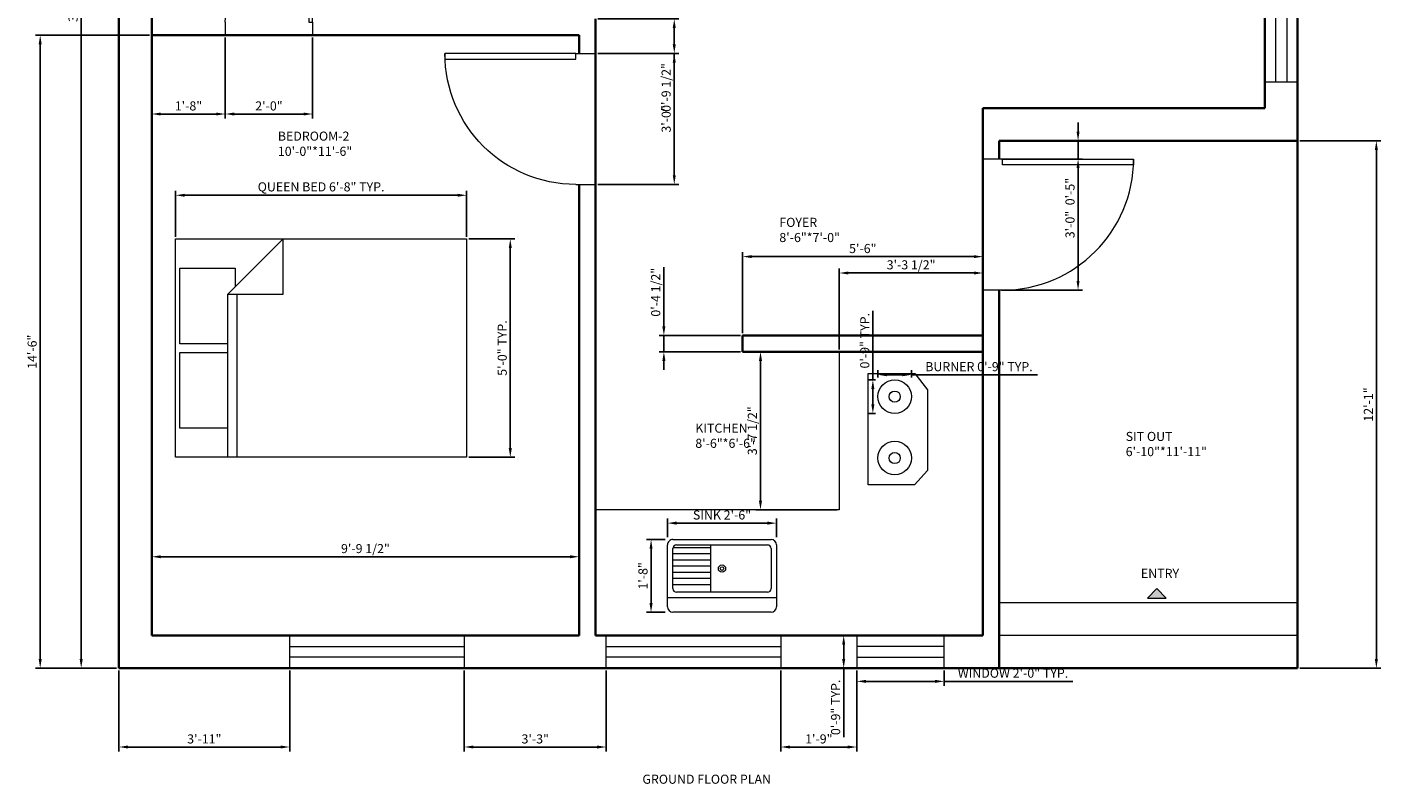
# Model space of a CAD drawing. Units: inches. Extents: x 2721 to 3093, y 1944 to 2371.
# Tile 1 of 2: x 2721 to 3093, y 1944 to 2152. Entities that reach past the tile are written whole.
import ezdxf

# ---------------------------------------------------------------- set-up
doc = ezdxf.new("R2010")
doc.units = ezdxf.units.IN
for name, color, linetype, lineweight in [('A-ANNO-DIMS', 2, 'Continuous', 18), ('A-ANNO-SYMB', 7, 'Continuous', 13), ('A-ANNO-SYMB-PATT', 7, 'Continuous', 13), ('A-ANNO-TEXT', 7, 'Continuous', 18), ('A-AREA-IDEN', 7, 'Continuous', 18), ('A-DOOR', 3, 'Continuous', 18), ('A-EQPM', 8, 'Continuous', 18), ('A-FLOR-CASE', 8, 'Continuous', 20), ('A-FLOR-FIXT', 8, 'Continuous', 18), ('A-FLOR-FIXT-PATT', 8, 'Continuous', 13), ('A-FLOR-STRS', 7, 'Continuous', 20), ('A-FURN', 9, 'Continuous', 18), ('A-GLAZ', 4, 'Continuous', 18), ('A-WALL', 7, 'Continuous', 35)]:
    doc.layers.add(name, color=color, linetype=linetype, lineweight=lineweight)
doc.styles.get("Standard").update_dxf_attribs({"font": 'arial.ttf'})
doc.dimstyles.new('ISO-25', dxfattribs={"dimtxt": 2.5, "dimasz": 2.5, "dimexe": 1.25, "dimexo": 0.625, "dimtad": 1, "dimdec": 1, "dimlunit": 3, "dimtxsty": 'Standard', "dimcen": 2.5, "dimadec": 0, "dimazin": 0, "dimtfac": 1, "dimtdec": 1, "dimtmove": 0, "dimatfit": 3, "dimfxl": 1, "dimarcsym": 0})

# ---------------------------------------------------------------- blocks, each defined once
blk = doc.blocks.new('*U2')
for p, q in [((0, 0), (0, -6)), ((40, 0), (40, -6))]:
    blk.add_line(p, q)
blk.add_lwpolyline([(0, 0), (0, 40), (1.75, 40), (1.75, 0)], close=True)
blk.add_arc((0, 0), 40, 0, 90)
blk = doc.blocks.new('Bed - Queen')
for p, q in [((0, -80.00003), (0, 0)), ((0, 0), (59.99999, 0)), ((59.99999, 0), (59.99999, -80.00003)), ((7.99999, -1.2), (28.79998, -1.2)), ((7.99999, -14.4), (7.99999, -1.2)), ((28.79998, -1.2), (28.79998, -14.4)), ((31.19999, -1.2), (51.99999, -1.2)), ((31.19999, -14.4), (31.19999, -1.2)), ((51.99999, -1.2), (51.99999, -16.4)), ((0, -14.4), (44.8, -14.4)), ((59.99999, -29.6), (44.8, -14.4)), ((44.8, -14.4), (44.8, -29.6)), ((44.8, -16.8), (0, -16.8)), ((51.99999, -16.4), (46.79936, -16.4)), ((44.8, -29.6), (59.99999, -29.6)), ((59.99999, -80.00003), (0, -80.00003))]:
    blk.add_line(p, q)
blk = doc.blocks.new('Sink-single - 30 in top')
blk.add_line((-15, -3.999996), (15, -3.999996))
for points in [[(-13.5, 0), (13.5, 0)], [(-15, -18.499996), (-15, -1.5)], [(15, -1.5), (15, -18.499996)], [(-13.5, -17.499996), (-13.5, -6.499996)], [(-12.5, -5.499996), (12.5, -5.499996)], [(13.5, -6.499996), (13.5, -17.499996)], [(12.5, -18.499996), (-12.5, -18.499996)], [(13.5, -19.999996), (-13.5, -19.999996)]]:
    blk.add_lwpolyline(points)
for radius in [1, 0.5]:
    blk.add_circle((0, -11.999996), radius)
for centre, radius, start, end in [((-13.5, -1.5), 1.5, 90, 180), ((13.5, -1.5), 1.5, 0, 90), ((-12.5, -6.499996), 1, 90, 180), ((12.5, -6.499996), 1, 0, 90), ((-13.5, -18.499996), 1.5, 180, 270), ((-12.5, -17.499996), 1, 180, 270), ((12.5, -17.499996), 1, 270, 0), ((13.5, -18.499996), 1.5, 270, 0)]:
    blk.add_arc(centre, radius, start, end)
blk = doc.blocks.new('*D7')
at = {"layer": 'A-ANNO-DIMS', "color": 0, "lineweight": -2, "transparency": 16777216}
for p, q in [((2745.17, 2336.18), (2734.17, 2336.18)), ((2735.42, 2333.68), (2735.42, 1978.68)), ((2745.17, 1976.18), (2734.17, 1976.18))]:
    blk.add_line(p, q, dxfattribs=at)
at = {"layer": 'A-ANNO-DIMS', "color": 0, "transparency": 16777216}
for points in [[(2735, 2333.68), (2735.84, 2333.68), (2735.42, 2336.18)], [(2735, 1978.68), (2735.84, 1978.68), (2735.42, 1976.18)]]:
    blk.add_solid(points, dxfattribs=at)
at = {"layer": 'Defpoints', "color": 0, "transparency": 16777216}
for p in [(2745.8, 2336.18), (2735.42, 1976.18), (2745.8, 1976.18)]:
    blk.add_point(p, dxfattribs=at)
at = {"layer": 'A-ANNO-DIMS', "color": 0, "transparency": 16777216, "insert": (2733.52, 2156.18), "char_height": 2.5, "attachment_point": 5, "rotation": 90}
blk.add_mtext("30'", dxfattribs=at)
blk = doc.blocks.new('WIN-48IN')
for p, q in [((0, 9), (48, 9)), ((0, 0), (0, 9)), ((48, 9), (48, 0)), ((0, 6), (48, 6)), ((48, 3), (0, 3)), ((48, 0), (0, 0))]:
    blk.add_line(p, q)
blk = doc.blocks.new('WIN-24IN')
for p, q in [((9, 24), (0, 24)), ((0, 24), (0, 0)), ((3, 24), (3, 0)), ((6, 0), (6, 24)), ((9, 0), (9, 24)), ((0, 0), (9, 0))]:
    blk.add_line(p, q)
blk = doc.blocks.new('COOKTOP-BURNER')
for radius in [4.62, 1.54]:
    blk.add_circle((4.62, 4.62), radius)
blk = doc.blocks.new('*D13')
at = {"layer": 'A-ANNO-DIMS', "color": 0, "lineweight": -2, "transparency": 16777216}
for p, q in [((2948.62, 1975.55), (2948.62, 1971.33)), ((2951.12, 1972.58), (2970.12, 1972.58)), ((2972.62, 1975.55), (2972.62, 1971.33)), ((2972.62, 1972.58), (3008, 1972.58))]:
    blk.add_line(p, q, dxfattribs=at)
at = {"layer": 'A-ANNO-DIMS', "color": 0, "transparency": 16777216}
for points in [[(2951.12, 1972.99), (2951.12, 1972.16), (2948.62, 1972.58)], [(2970.12, 1972.99), (2970.12, 1972.16), (2972.62, 1972.58)]]:
    blk.add_solid(points, dxfattribs=at)
at = {"layer": 'Defpoints', "color": 0, "transparency": 16777216}
for p in [(2948.62, 1976.18), (2972.62, 1976.18), (2972.62, 1972.58)]:
    blk.add_point(p, dxfattribs=at)
at = {"layer": 'A-ANNO-DIMS', "color": 0, "transparency": 16777216, "insert": (2991.56, 1974.5), "char_height": 2.5, "attachment_point": 5}
blk.add_mtext('WINDOW 2\'-0" TYP.', dxfattribs=at)
blk = doc.blocks.new('*D14')
at = {"layer": 'A-ANNO-DIMS', "color": 0, "lineweight": -2, "transparency": 16777216}
for p, q in [((2947.99, 1985.18), (2943.77, 1985.18)), ((2945.02, 1982.68), (2945.02, 1978.68)), ((2947.99, 1976.18), (2943.77, 1976.18)), ((2945.02, 1976.18), (2945.02, 1957.19))]:
    blk.add_line(p, q, dxfattribs=at)
at = {"layer": 'A-ANNO-DIMS', "color": 0, "transparency": 16777216}
for points in [[(2944.6, 1982.68), (2945.43, 1982.68), (2945.02, 1985.18)], [(2944.6, 1978.68), (2945.43, 1978.68), (2945.02, 1976.18)]]:
    blk.add_solid(points, dxfattribs=at)
at = {"layer": 'Defpoints', "color": 0, "transparency": 16777216}
for p in [(2948.62, 1985.18), (2945.02, 1976.18), (2948.62, 1976.18)]:
    blk.add_point(p, dxfattribs=at)
at = {"layer": 'A-ANNO-DIMS', "color": 0, "transparency": 16777216, "insert": (2943.12, 1965.43), "char_height": 2.5, "attachment_point": 5, "rotation": 90}
blk.add_mtext('0\'-9" TYP.', dxfattribs=at)
blk = doc.blocks.new('*D15')
at = {"layer": 'A-ANNO-DIMS', "color": 0, "lineweight": -2, "transparency": 16777216}
for p, q in [((2761.37, 2094.81), (2761.37, 2107.44)), ((2841.37, 2094.81), (2841.37, 2107.44)), ((2838.87, 2106.19), (2763.87, 2106.19))]:
    blk.add_line(p, q, dxfattribs=at)
at = {"layer": 'A-ANNO-DIMS', "color": 0, "transparency": 16777216}
for points in [[(2763.87, 2106.61), (2763.87, 2105.77), (2761.37, 2106.19)], [(2838.87, 2106.61), (2838.87, 2105.77), (2841.37, 2106.19)]]:
    blk.add_solid(points, dxfattribs=at)
at = {"layer": 'Defpoints', "color": 0, "transparency": 16777216}
for p in [(2761.37, 2106.19), (2761.37, 2094.19), (2841.37, 2094.19)]:
    blk.add_point(p, dxfattribs=at)
at = {"layer": 'A-ANNO-DIMS', "color": 0, "transparency": 16777216, "insert": (2801.37, 2108.18), "char_height": 2.5, "attachment_point": 5}
blk.add_mtext('QUEEN BED 6\'-8" TYP.', dxfattribs=at)
blk = doc.blocks.new('*D16')
at = {"layer": 'A-ANNO-DIMS', "color": 0, "lineweight": -2, "transparency": 16777216}
for p, q in [((2842, 2094.19), (2854.62, 2094.19)), ((2853.37, 2036.69), (2853.37, 2091.69)), ((2842, 2034.19), (2854.62, 2034.19))]:
    blk.add_line(p, q, dxfattribs=at)
at = {"layer": 'A-ANNO-DIMS', "color": 0, "transparency": 16777216}
for points in [[(2852.95, 2091.69), (2853.79, 2091.69), (2853.37, 2094.19)], [(2852.95, 2036.69), (2853.79, 2036.69), (2853.37, 2034.19)]]:
    blk.add_solid(points, dxfattribs=at)
at = {"layer": 'Defpoints', "color": 0, "transparency": 16777216}
for p in [(2841.37, 2094.19), (2853.37, 2094.19), (2841.37, 2034.19)]:
    blk.add_point(p, dxfattribs=at)
at = {"layer": 'A-ANNO-DIMS', "color": 0, "transparency": 16777216, "insert": (2851.47, 2064.19), "char_height": 2.5, "attachment_point": 5, "rotation": 90}
blk.add_mtext('5\'-0" TYP.', dxfattribs=at)
blk = doc.blocks.new('*D19')
at = {"layer": 'A-ANNO-DIMS', "color": 0, "lineweight": -2, "transparency": 16777216}
for p, q in [((2954.43, 2056.09), (2954.43, 2058.1)), ((2963.66, 2056.09), (2963.66, 2058.1)), ((2956.93, 2056.85), (2961.16, 2056.85)), ((2963.66, 2056.85), (2998.26, 2056.85))]:
    blk.add_line(p, q, dxfattribs=at)
at = {"layer": 'A-ANNO-DIMS', "color": 0, "transparency": 16777216}
for points in [[(2956.93, 2057.27), (2956.93, 2056.44), (2954.43, 2056.85)], [(2961.16, 2057.27), (2961.16, 2056.44), (2963.66, 2056.85)]]:
    blk.add_solid(points, dxfattribs=at)
at = {"layer": 'Defpoints', "color": 0, "transparency": 16777216}
for p in [(2954.43, 2055.47), (2963.66, 2056.85), (2963.66, 2055.47)]:
    blk.add_point(p, dxfattribs=at)
at = {"layer": 'A-ANNO-DIMS', "color": 0, "transparency": 16777216, "insert": (2982.21, 2058.76), "char_height": 2.5, "attachment_point": 5}
blk.add_mtext('BURNER 0\'-9" TYP.', dxfattribs=at)
blk = doc.blocks.new('*D20')
at = {"layer": 'A-ANNO-DIMS', "color": 0, "lineweight": -2, "transparency": 16777216}
for p, q in [((2953.04, 2055.47), (2953.04, 2074.46)), ((2953.8, 2055.47), (2951.79, 2055.47)), ((2953.04, 2048.73), (2953.04, 2052.97)), ((2953.8, 2046.23), (2951.79, 2046.23))]:
    blk.add_line(p, q, dxfattribs=at)
at = {"layer": 'A-ANNO-DIMS', "color": 0, "transparency": 16777216}
for points in [[(2952.62, 2052.97), (2953.46, 2052.97), (2953.04, 2055.47)], [(2952.62, 2048.73), (2953.46, 2048.73), (2953.04, 2046.23)]]:
    blk.add_solid(points, dxfattribs=at)
at = {"layer": 'Defpoints', "color": 0, "transparency": 16777216}
for p in [(2953.04, 2055.47), (2954.43, 2055.47), (2954.43, 2046.23)]:
    blk.add_point(p, dxfattribs=at)
at = {"layer": 'A-ANNO-DIMS', "color": 0, "transparency": 16777216, "insert": (2951.14, 2066.21), "char_height": 2.5, "attachment_point": 5, "rotation": 90}
blk.add_mtext('0\'-9" TYP.', dxfattribs=at)
blk = doc.blocks.new('*D21')
at = {"layer": 'A-ANNO-DIMS', "color": 0, "lineweight": -2, "transparency": 16777216}
for p, q in [((2896.57, 2012.2), (2896.57, 2017.32)), ((2926.57, 2012.2), (2926.57, 2017.32)), ((2924.07, 2016.07), (2899.07, 2016.07))]:
    blk.add_line(p, q, dxfattribs=at)
at = {"layer": 'A-ANNO-DIMS', "color": 0, "transparency": 16777216}
for points in [[(2899.07, 2016.49), (2899.07, 2015.65), (2896.57, 2016.07)], [(2924.07, 2016.49), (2924.07, 2015.65), (2926.57, 2016.07)]]:
    blk.add_solid(points, dxfattribs=at)
at = {"layer": 'Defpoints', "color": 0, "transparency": 16777216}
for p in [(2896.57, 2016.07), (2896.57, 2011.57), (2926.57, 2011.57)]:
    blk.add_point(p, dxfattribs=at)
at = {"layer": 'A-ANNO-DIMS', "color": 0, "transparency": 16777216, "insert": (2911.57, 2017.99), "char_height": 2.5, "attachment_point": 5}
blk.add_mtext('SINK 2\'-6"', dxfattribs=at)
blk = doc.blocks.new('*D22')
at = {"layer": 'A-ANNO-DIMS', "color": 0, "lineweight": -2, "transparency": 16777216}
for p, q in [((2895.94, 2011.57), (2890.82, 2011.57)), ((2892.07, 2009.07), (2892.07, 1994.07)), ((2895.94, 1991.57), (2890.82, 1991.57))]:
    blk.add_line(p, q, dxfattribs=at)
at = {"layer": 'A-ANNO-DIMS', "color": 0, "transparency": 16777216}
for points in [[(2891.65, 2009.07), (2892.48, 2009.07), (2892.07, 2011.57)], [(2891.65, 1994.07), (2892.48, 1994.07), (2892.07, 1991.57)]]:
    blk.add_solid(points, dxfattribs=at)
at = {"layer": 'Defpoints', "color": 0, "transparency": 16777216}
for p in [(2896.57, 2011.57), (2892.07, 1991.57), (2896.57, 1991.57)]:
    blk.add_point(p, dxfattribs=at)
at = {"layer": 'A-ANNO-DIMS', "color": 0, "transparency": 16777216, "insert": (2890.17, 2001.57), "char_height": 2.5, "attachment_point": 5, "rotation": 90}
blk.add_mtext('1\'-8"', dxfattribs=at)
blk = doc.blocks.new('*D25')
at = {"layer": 'A-ANNO-DIMS', "color": 0, "lineweight": -2, "transparency": 16777216}
for p, q in [((2745.8, 1975.55), (2745.8, 1953.28)), ((2792.73, 1975.55), (2792.73, 1953.28)), ((2790.23, 1954.53), (2748.3, 1954.53))]:
    blk.add_line(p, q, dxfattribs=at)
at = {"layer": 'A-ANNO-DIMS', "color": 0, "transparency": 16777216}
for points in [[(2748.3, 1954.94), (2748.3, 1954.11), (2745.8, 1954.53)], [(2790.23, 1954.94), (2790.23, 1954.11), (2792.73, 1954.53)]]:
    blk.add_solid(points, dxfattribs=at)
at = {"layer": 'Defpoints', "color": 0, "transparency": 16777216}
for p in [(2745.8, 1976.18), (2792.73, 1976.18), (2745.8, 1954.53)]:
    blk.add_point(p, dxfattribs=at)
at = {"layer": 'A-ANNO-DIMS', "color": 0, "transparency": 16777216, "insert": (2769.26, 1956.43), "char_height": 2.5, "attachment_point": 5}
blk.add_mtext('3\'-11"', dxfattribs=at)
blk = doc.blocks.new('*D26')
at = {"layer": 'A-ANNO-DIMS', "color": 0, "lineweight": -2, "transparency": 16777216}
for p, q in [((2840.73, 1975.55), (2840.73, 1953.28)), ((2879.73, 1975.55), (2879.73, 1953.28)), ((2877.23, 1954.53), (2843.23, 1954.53))]:
    blk.add_line(p, q, dxfattribs=at)
at = {"layer": 'A-ANNO-DIMS', "color": 0, "transparency": 16777216}
for points in [[(2843.23, 1954.94), (2843.23, 1954.11), (2840.73, 1954.53)], [(2877.23, 1954.94), (2877.23, 1954.11), (2879.73, 1954.53)]]:
    blk.add_solid(points, dxfattribs=at)
at = {"layer": 'Defpoints', "color": 0, "transparency": 16777216}
for p in [(2840.73, 1976.18), (2879.73, 1976.18), (2840.73, 1954.53)]:
    blk.add_point(p, dxfattribs=at)
at = {"layer": 'A-ANNO-DIMS', "color": 0, "transparency": 16777216, "insert": (2860.23, 1956.43), "char_height": 2.5, "attachment_point": 5}
blk.add_mtext('3\'-3"', dxfattribs=at)
blk = doc.blocks.new('*D27')
at = {"layer": 'A-ANNO-DIMS', "color": 0, "lineweight": -2, "transparency": 16777216}
for p, q in [((2927.73, 1975.55), (2927.73, 1953.28)), ((2948.62, 1975.55), (2948.62, 1953.28)), ((2946.12, 1954.53), (2930.23, 1954.53))]:
    blk.add_line(p, q, dxfattribs=at)
at = {"layer": 'A-ANNO-DIMS', "color": 0, "transparency": 16777216}
for points in [[(2930.23, 1954.94), (2930.23, 1954.11), (2927.73, 1954.53)], [(2946.12, 1954.94), (2946.12, 1954.11), (2948.62, 1954.53)]]:
    blk.add_solid(points, dxfattribs=at)
at = {"layer": 'Defpoints', "color": 0, "transparency": 16777216}
for p in [(2927.73, 1976.18), (2948.62, 1976.18), (2927.73, 1954.53)]:
    blk.add_point(p, dxfattribs=at)
at = {"layer": 'A-ANNO-DIMS', "color": 0, "transparency": 16777216, "insert": (2938.18, 1956.43), "char_height": 2.5, "attachment_point": 5}
blk.add_mtext('1\'-9"', dxfattribs=at)
blk = doc.blocks.new('*D32')
at = {"layer": 'A-ANNO-DIMS', "color": 0, "lineweight": -2, "transparency": 16777216}
for p, q in [((2988.42, 2116.15), (3010.7, 2116.15)), ((3009.45, 2113.65), (3009.45, 2082.65)), ((2988.42, 2080.15), (3010.7, 2080.15))]:
    blk.add_line(p, q, dxfattribs=at)
at = {"layer": 'A-ANNO-DIMS', "color": 0, "transparency": 16777216}
for points in [[(3009.03, 2113.65), (3009.86, 2113.65), (3009.45, 2116.15)], [(3009.03, 2082.65), (3009.86, 2082.65), (3009.45, 2080.15)]]:
    blk.add_solid(points, dxfattribs=at)
at = {"layer": 'Defpoints', "color": 0, "transparency": 16777216}
for p in [(2987.8, 2116.15), (2987.8, 2080.15), (3009.45, 2080.15)]:
    blk.add_point(p, dxfattribs=at)
at = {"layer": 'A-ANNO-DIMS', "color": 0, "transparency": 16777216, "insert": (3007.55, 2098.15), "char_height": 2.5, "attachment_point": 5, "rotation": 90}
blk.add_mtext('3\'-0"', dxfattribs=at)
blk = doc.blocks.new('*D33')
at = {"layer": 'A-ANNO-DIMS', "color": 0, "lineweight": -2, "transparency": 16777216}
for p, q in [((2775.03, 2149.55), (2775.03, 2127.28)), ((2799.03, 2149.55), (2799.03, 2127.28)), ((2796.53, 2128.53), (2777.53, 2128.53))]:
    blk.add_line(p, q, dxfattribs=at)
at = {"layer": 'A-ANNO-DIMS', "color": 0, "transparency": 16777216}
for points in [[(2777.53, 2128.94), (2777.53, 2128.11), (2775.03, 2128.53)], [(2796.53, 2128.94), (2796.53, 2128.11), (2799.03, 2128.53)]]:
    blk.add_solid(points, dxfattribs=at)
at = {"layer": 'Defpoints', "color": 0, "transparency": 16777216}
for p in [(2775.03, 2150.18), (2799.03, 2150.18), (2775.03, 2128.53)]:
    blk.add_point(p, dxfattribs=at)
at = {"layer": 'A-ANNO-DIMS', "color": 0, "transparency": 16777216, "insert": (2787.03, 2130.43), "char_height": 2.5, "attachment_point": 5}
blk.add_mtext('2\'-0"', dxfattribs=at)
blk = doc.blocks.new('*D37')
at = {"layer": 'A-ANNO-DIMS', "color": 0, "lineweight": -2, "transparency": 16777216}
for p, q in [((2877.42, 2145.18), (2899.7, 2145.18)), ((2898.45, 2142.68), (2898.45, 2111.68)), ((2877.42, 2109.18), (2899.7, 2109.18))]:
    blk.add_line(p, q, dxfattribs=at)
at = {"layer": 'A-ANNO-DIMS', "color": 0, "transparency": 16777216}
for points in [[(2898.03, 2142.68), (2898.86, 2142.68), (2898.45, 2145.18)], [(2898.03, 2111.68), (2898.86, 2111.68), (2898.45, 2109.18)]]:
    blk.add_solid(points, dxfattribs=at)
at = {"layer": 'Defpoints', "color": 0, "transparency": 16777216}
for p in [(2876.8, 2145.18), (2876.8, 2109.18), (2898.45, 2109.18)]:
    blk.add_point(p, dxfattribs=at)
at = {"layer": 'A-ANNO-DIMS', "color": 0, "transparency": 16777216, "insert": (2896.55, 2127.18), "char_height": 2.5, "attachment_point": 5, "rotation": 90}
blk.add_mtext('3\'-0"', dxfattribs=at)
blk = doc.blocks.new('*D38')
at = {"layer": 'A-ANNO-DIMS', "color": 0, "lineweight": -2, "transparency": 16777216}
for p, q in [((3070.42, 2121.18), (3092.7, 2121.18)), ((3091.45, 2118.68), (3091.45, 1978.68)), ((3070.42, 1976.18), (3092.7, 1976.18))]:
    blk.add_line(p, q, dxfattribs=at)
at = {"layer": 'A-ANNO-DIMS', "color": 0, "transparency": 16777216}
for points in [[(3091.03, 2118.68), (3091.86, 2118.68), (3091.45, 2121.18)], [(3091.03, 1978.68), (3091.86, 1978.68), (3091.45, 1976.18)]]:
    blk.add_solid(points, dxfattribs=at)
at = {"layer": 'Defpoints', "color": 0, "transparency": 16777216}
for p in [(3069.8, 2121.18), (3069.8, 1976.18), (3091.45, 1976.18)]:
    blk.add_point(p, dxfattribs=at)
at = {"layer": 'A-ANNO-DIMS', "color": 0, "transparency": 16777216, "insert": (3089.57, 2048.68), "char_height": 2.5, "attachment_point": 5, "rotation": 90}
blk.add_mtext('12\'-1"', dxfattribs=at)
blk = doc.blocks.new('*D39')
at = {"layer": 'A-ANNO-DIMS', "color": 0, "lineweight": -2, "transparency": 16777216}
for p, q in [((2754.8, 2149.55), (2754.8, 2127.28)), ((2775.03, 2149.55), (2775.03, 2127.28)), ((2772.53, 2128.53), (2757.3, 2128.53))]:
    blk.add_line(p, q, dxfattribs=at)
at = {"layer": 'A-ANNO-DIMS', "color": 0, "transparency": 16777216}
for points in [[(2757.3, 2128.94), (2757.3, 2128.11), (2754.8, 2128.53)], [(2772.53, 2128.94), (2772.53, 2128.11), (2775.03, 2128.53)]]:
    blk.add_solid(points, dxfattribs=at)
at = {"layer": 'Defpoints', "color": 0, "transparency": 16777216}
for p in [(2754.8, 2150.18), (2775.03, 2150.18), (2754.8, 2128.53)]:
    blk.add_point(p, dxfattribs=at)
at = {"layer": 'A-ANNO-DIMS', "color": 0, "transparency": 16777216, "insert": (2764.91, 2130.43), "char_height": 2.5, "attachment_point": 5}
blk.add_mtext('1\'-8"', dxfattribs=at)
blk = doc.blocks.new('*D40')
at = {"layer": 'A-ANNO-DIMS', "color": 0, "lineweight": -2, "transparency": 16777216}
for p, q in [((3009.45, 2123.68), (3009.45, 2126.18)), ((2988.42, 2121.18), (3010.7, 2121.18)), ((3009.45, 2121.18), (3009.45, 2116.15)), ((2988.42, 2116.15), (3010.7, 2116.15)), ((3009.45, 2113.65), (3009.45, 2103.26))]:
    blk.add_line(p, q, dxfattribs=at)
at = {"layer": 'A-ANNO-DIMS', "color": 0, "transparency": 16777216}
for points in [[(3009.03, 2123.68), (3009.86, 2123.68), (3009.45, 2121.18)], [(3009.03, 2113.65), (3009.86, 2113.65), (3009.45, 2116.15)]]:
    blk.add_solid(points, dxfattribs=at)
at = {"layer": 'Defpoints', "color": 0, "transparency": 16777216}
for p in [(2987.8, 2121.18), (2987.8, 2116.15), (3009.45, 2116.15)]:
    blk.add_point(p, dxfattribs=at)
at = {"layer": 'A-ANNO-DIMS', "color": 0, "transparency": 16777216, "insert": (3007.55, 2107.21), "char_height": 2.5, "attachment_point": 5, "rotation": 90}
blk.add_mtext('0\'-5"', dxfattribs=at)
blk = doc.blocks.new('*D41')
at = {"layer": 'A-ANNO-DIMS', "color": 0, "lineweight": -2, "transparency": 16777216}
for p, q in [((2917.24, 2068.3), (2917.24, 2090.58)), ((2919.74, 2089.33), (2980.8, 2089.33)), ((2983.3, 2068.3), (2983.3, 2090.58))]:
    blk.add_line(p, q, dxfattribs=at)
at = {"layer": 'A-ANNO-DIMS', "color": 0, "transparency": 16777216}
for points in [[(2919.74, 2089.74), (2919.74, 2088.91), (2917.24, 2089.33)], [(2980.8, 2089.74), (2980.8, 2088.91), (2983.3, 2089.33)]]:
    blk.add_solid(points, dxfattribs=at)
at = {"layer": 'Defpoints', "color": 0, "transparency": 16777216}
for p in [(2983.3, 2089.33), (2917.24, 2067.68), (2983.3, 2067.68)]:
    blk.add_point(p, dxfattribs=at)
at = {"layer": 'A-ANNO-DIMS', "color": 0, "transparency": 16777216, "insert": (2950.27, 2091.23), "char_height": 2.5, "attachment_point": 5}
blk.add_mtext('5\'-6"', dxfattribs=at)
blk = doc.blocks.new('*D42')
at = {"layer": 'A-ANNO-DIMS', "color": 0, "lineweight": -2, "transparency": 16777216}
for p, q in [((2895.59, 2070.18), (2895.59, 2086.4)), ((2916.61, 2067.68), (2894.34, 2067.68)), ((2895.59, 2063.18), (2895.59, 2067.68)), ((2916.61, 2063.18), (2894.34, 2063.18)), ((2895.59, 2060.68), (2895.59, 2058.18))]:
    blk.add_line(p, q, dxfattribs=at)
at = {"layer": 'A-ANNO-DIMS', "color": 0, "transparency": 16777216}
for points in [[(2895.17, 2070.18), (2896.01, 2070.18), (2895.59, 2067.68)], [(2895.17, 2060.68), (2896.01, 2060.68), (2895.59, 2063.18)]]:
    blk.add_solid(points, dxfattribs=at)
at = {"layer": 'Defpoints', "color": 0, "transparency": 16777216}
for p in [(2895.59, 2067.68), (2917.24, 2067.68), (2917.24, 2063.18)]:
    blk.add_point(p, dxfattribs=at)
at = {"layer": 'A-ANNO-DIMS', "color": 0, "transparency": 16777216, "insert": (2893.67, 2079.54), "char_height": 2.5, "attachment_point": 5, "rotation": 90}
blk.add_mtext('0\'-4 1/2"', dxfattribs=at)
blk = doc.blocks.new('*D46')
at = {"layer": 'A-ANNO-DIMS', "color": 0, "lineweight": -2, "transparency": 16777216}
for p, q in [((2877.42, 2154.68), (2899.7, 2154.68)), ((2898.45, 2152.18), (2898.45, 2147.68)), ((2877.42, 2145.18), (2899.7, 2145.18)), ((2898.45, 2145.18), (2898.45, 2128.96))]:
    blk.add_line(p, q, dxfattribs=at)
at = {"layer": 'A-ANNO-DIMS', "color": 0, "transparency": 16777216}
for points in [[(2898.03, 2152.18), (2898.86, 2152.18), (2898.45, 2154.68)], [(2898.03, 2147.68), (2898.86, 2147.68), (2898.45, 2145.18)]]:
    blk.add_solid(points, dxfattribs=at)
at = {"layer": 'Defpoints', "color": 0, "transparency": 16777216}
for p in [(2876.8, 2154.68), (2876.8, 2145.18), (2898.45, 2145.18)]:
    blk.add_point(p, dxfattribs=at)
at = {"layer": 'A-ANNO-DIMS', "color": 0, "transparency": 16777216, "insert": (2896.53, 2135.82), "char_height": 2.5, "attachment_point": 5, "rotation": 90}
blk.add_mtext('0\'-9 1/2"', dxfattribs=at)
blk = doc.blocks.new('*D47')
at = {"layer": 'A-ANNO-DIMS', "color": 0, "lineweight": -2, "transparency": 16777216}
for p, q in [((2754.17, 2150.18), (2722.9, 2150.18)), ((2724.15, 2147.68), (2724.15, 1978.68)), ((2745.17, 1976.18), (2722.9, 1976.18))]:
    blk.add_line(p, q, dxfattribs=at)
at = {"layer": 'A-ANNO-DIMS', "color": 0, "transparency": 16777216}
for points in [[(2723.73, 2147.68), (2724.56, 2147.68), (2724.15, 2150.18)], [(2723.73, 1978.68), (2724.56, 1978.68), (2724.15, 1976.18)]]:
    blk.add_solid(points, dxfattribs=at)
at = {"layer": 'Defpoints', "color": 0, "transparency": 16777216}
for p in [(2754.8, 2150.18), (2724.15, 1976.18), (2745.8, 1976.18)]:
    blk.add_point(p, dxfattribs=at)
at = {"layer": 'A-ANNO-DIMS', "color": 0, "transparency": 16777216, "insert": (2722.25, 2063.18), "char_height": 2.5, "attachment_point": 5, "rotation": 90}
blk.add_mtext('14\'-6"', dxfattribs=at)
blk = doc.blocks.new('*D48')
at = {"layer": 'A-ANNO-DIMS', "color": 0, "lineweight": -2, "transparency": 16777216}
for p, q in [((2754.8, 1985.8), (2754.8, 2008.08)), ((2757.3, 2006.83), (2869.8, 2006.83)), ((2872.3, 1985.8), (2872.3, 2008.08))]:
    blk.add_line(p, q, dxfattribs=at)
at = {"layer": 'A-ANNO-DIMS', "color": 0, "transparency": 16777216}
for points in [[(2757.3, 2007.24), (2757.3, 2006.41), (2754.8, 2006.83)], [(2869.8, 2007.24), (2869.8, 2006.41), (2872.3, 2006.83)]]:
    blk.add_solid(points, dxfattribs=at)
at = {"layer": 'Defpoints', "color": 0, "transparency": 16777216}
for p in [(2872.3, 2006.83), (2754.8, 1985.18), (2872.3, 1985.18)]:
    blk.add_point(p, dxfattribs=at)
at = {"layer": 'A-ANNO-DIMS', "color": 0, "transparency": 16777216, "insert": (2813.55, 2008.75), "char_height": 2.5, "attachment_point": 5}
blk.add_mtext('9\'-9 1/2"', dxfattribs=at)
blk = doc.blocks.new('*D50')
at = {"layer": 'A-ANNO-DIMS', "color": 0, "lineweight": -2, "transparency": 16777216}
for p, q in [((2943.8, 2063.8), (2943.8, 2086.08)), ((2946.3, 2084.83), (2980.8, 2084.83)), ((2983.3, 2063.8), (2983.3, 2086.08))]:
    blk.add_line(p, q, dxfattribs=at)
at = {"layer": 'A-ANNO-DIMS', "color": 0, "transparency": 16777216}
for points in [[(2946.3, 2085.24), (2946.3, 2084.41), (2943.8, 2084.83)], [(2980.8, 2085.24), (2980.8, 2084.41), (2983.3, 2084.83)]]:
    blk.add_solid(points, dxfattribs=at)
at = {"layer": 'Defpoints', "color": 0, "transparency": 16777216}
for p in [(2983.3, 2084.83), (2943.8, 2063.18), (2983.3, 2063.18)]:
    blk.add_point(p, dxfattribs=at)
at = {"layer": 'A-ANNO-DIMS', "color": 0, "transparency": 16777216, "insert": (2963.55, 2086.75), "char_height": 2.5, "attachment_point": 5}
blk.add_mtext('3\'-3 1/2"', dxfattribs=at)
blk = doc.blocks.new('*D51')
at = {"layer": 'A-ANNO-DIMS', "color": 0, "lineweight": -2, "transparency": 16777216}
for p, q in [((2943.17, 2063.18), (2920.9, 2063.18)), ((2922.15, 2022.24), (2922.15, 2060.68)), ((2943.17, 2019.74), (2920.9, 2019.74))]:
    blk.add_line(p, q, dxfattribs=at)
at = {"layer": 'A-ANNO-DIMS', "color": 0, "transparency": 16777216}
for points in [[(2921.73, 2060.68), (2922.57, 2060.68), (2922.15, 2063.18)], [(2921.73, 2022.24), (2922.57, 2022.24), (2922.15, 2019.74)]]:
    blk.add_solid(points, dxfattribs=at)
at = {"layer": 'Defpoints', "color": 0, "transparency": 16777216}
for p in [(2922.15, 2063.18), (2943.8, 2063.18), (2943.8, 2019.74)]:
    blk.add_point(p, dxfattribs=at)
at = {"layer": 'A-ANNO-DIMS', "color": 0, "transparency": 16777216, "insert": (2920.23, 2041.46), "char_height": 2.5, "attachment_point": 5, "rotation": 90}
blk.add_mtext('3\'-7 1/2"', dxfattribs=at)

msp = doc.modelspace()

# ---------------------------------------------------------------- hatches: boundary and pattern name
at = {"layer": 'A-ANNO-SYMB-PATT'}
h = msp.add_hatch(color=256, dxfattribs=at)
h.dxf.hatch_style = 1
h.paths.add_polyline_path([(3031.12, 1998.13), (3028.57, 1995.45), (3033.66, 1995.45)])
at = {"layer": 'A-FLOR-FIXT-PATT'}
h = msp.add_hatch(dxfattribs=at)
h.set_pattern_fill('ANSI31', color=256, scale=0.535433, angle=-45, style=0)
h.paths.add_polyline_path([(2898.07, 1997.91), (2908.38, 1997.91), (2908.38, 2009.81), (2898.07, 2009.81)])

# ---------------------------------------------------------------- linework, layer by layer
at = {"layer": 'A-ANNO-SYMB'}
for p, q in [((3028.57, 1995.45), (3031.12, 1998.13)), ((3028.57, 1995.45), (3033.66, 1995.45)), ((3031.12, 1998.13), (3033.66, 1995.45))]:
    msp.add_line(p, q, dxfattribs=at)
at = {"layer": 'A-EQPM'}
for p, q in [((2964.55, 2057.18), (2968.02, 2052.71)), ((2964.51, 2026.57), (2968.02, 2030.58))]:
    msp.add_line(p, q, dxfattribs=at)
for points in [[(2964.51, 2026.57), (2951.78, 2026.57), (2951.78, 2057.18), (2964.55, 2057.18)], [(2968.02, 2052.71), (2968.02, 2030.58)]]:
    msp.add_lwpolyline(points, dxfattribs=at)
at = {"layer": 'A-FLOR-CASE'}
for p, q in [((2943.8, 2063.18), (2943.8, 2019.74)), ((2943.8, 2019.74), (2876.8, 2019.74))]:
    msp.add_line(p, q, dxfattribs=at)
at = {"layer": 'A-FLOR-FIXT'}
msp.add_line((2908.38, 2010.07), (2908.38, 1997.07), dxfattribs=at)
at = {"layer": 'A-FLOR-STRS'}
for p, q in [((3069.8, 1994.18), (2987.8, 1994.18)), ((3069.8, 1985.18), (2987.8, 1985.18))]:
    msp.add_line(p, q, dxfattribs=at)
at = {"layer": 'A-WALL'}
for p, q in [((2745.8, 1976.18), (2745.8, 2336.18)), ((3069.8, 2336.18), (3069.8, 1976.18)), ((2754.8, 1985.18), (2754.8, 2327.18)), ((3060.8, 2327.18), (3060.8, 2130.18)), ((2876.8, 2154.68), (2876.8, 1985.18)), ((2754.8, 2150.18), (2872.3, 2150.18)), ((2872.3, 2150.18), (2872.3, 2145.18)), ((2983.3, 2130.18), (3060.8, 2130.18)), ((2983.3, 2130.18), (2983.3, 1985.18)), ((2987.8, 2121.18), (2987.8, 2116.15)), ((2987.8, 2121.18), (3069.8, 2121.18)), ((2872.3, 2109.18), (2872.3, 1985.18)), ((2987.8, 2080.15), (2987.8, 1976.18)), ((2983.3, 2067.68), (2917.24, 2067.68)), ((2917.24, 2067.68), (2917.24, 2063.18)), ((2983.3, 2063.18), (2917.24, 2063.18)), ((2872.3, 1985.18), (2754.8, 1985.18)), ((2983.3, 1985.18), (2876.8, 1985.18)), ((3069.8, 1976.18), (2745.8, 1976.18))]:
    msp.add_line(p, q, dxfattribs=at)

# ---------------------------------------------------------------- block references
at = {"layer": 'A-DOOR', "xscale": -0.6, "yscale": 0.6, "zscale": 0.6}
msp.add_blockref('*U2', (2799.03, 2153.78), dxfattribs=at)
at = {"layer": 'A-DOOR', "yscale": 0.9, "zscale": 0.9}
for p, xscale, rotation in [((2871.4, 2145.18), -0.9, 90), ((2988.7, 2116.15), 0.9, 270)]:
    msp.add_blockref('*U2', p, dxfattribs=dict(at, xscale=xscale, rotation=rotation))
at = {"layer": 'A-EQPM'}
for p in [(2954.43, 2046.23), (2954.43, 2029.34)]:
    msp.add_blockref('COOKTOP-BURNER', p, dxfattribs=at)
at = {"layer": 'A-FLOR-FIXT', "rotation": 180}
msp.add_blockref('Sink-single - 30 in top', (2911.57, 1991.57), dxfattribs=at)
at = {"layer": 'A-FURN', "rotation": 90}
msp.add_blockref('Bed - Queen', (2761.37, 2034.19), dxfattribs=at)
at = {"layer": 'A-GLAZ'}
for name, p, rotation in [('WIN-48IN', (3069.8, 2137.31), 90.00000000000276), ('WIN-24IN', (2948.62, 1985.18), 269.9999999999943)]:
    msp.add_blockref(name, p, dxfattribs=dict(at, rotation=rotation))
for p in [(2792.73, 1976.18), (2879.73, 1976.18)]:
    msp.add_blockref('WIN-48IN', p, dxfattribs=at)

# ---------------------------------------------------------------- texts
at = {"layer": 'A-ANNO-TEXT', "char_height": 2.5, "attachment_point": 1}
for s, width, insert in [('ENTRY', 30.8668, (3026.72, 2003.51)), ('GROUND FLOOR PLAN', 281.0188, (2889.69, 1946.93))]:
    msp.add_mtext_dynamic_manual_height_columns(s, width=width, gutter_width=12.5, heights=[0], dxfattribs=dict(at, insert=insert))
at = {"layer": 'A-AREA-IDEN', "char_height": 2.5, "attachment_point": 1}
for s, width, insert in [('BEDROOM-2\\P10\'-0"*11\'-6"', 63.9317, (2789.48, 2123.7)), ('FOYER\\P8\'-6"*7\'-0"', 60.4833, (2927.33, 2100)), ('KITCHEN\\P8\'-6"*6\'-6"', 48.4763, (2904.23, 2043.43)), ('SIT OUT\\P6\'-10"*11\'-11"', 49.8956, (3022.54, 2041.15))]:
    msp.add_mtext_dynamic_manual_height_columns(s, width=width, gutter_width=12.5, heights=[0], dxfattribs=dict(at, insert=insert))

# ---------------------------------------------------------------- dimensions: what is measured, and where the dimension line sits
at = {"layer": 'A-ANNO-DIMS'}
for base, p1, p2, angle, override, picture, middle in [((2735.42, 1976.18), (2745.8, 2336.18), (2745.8, 1976.18), 90, {"dimclrd": 0, "dimclre": 0, "dimclrt": 0}, '*D7', (2733.52, 2156.18)), ((2898.45, 2145.18), (2876.8, 2154.68), (2876.8, 2145.18), 270, {"dimdec": 1, "dimlfac": 1, "dimrnd": 0, "dimzin": 1, "dimdsep": 46, "dimlunit": 4, "dimfrac": 2}, '*D46', (2896.53, 2135.82)), ((2724.15, 1976.18), (2754.8, 2150.18), (2745.8, 1976.18), 90, {"dimdec": 1, "dimlfac": 1, "dimrnd": 0, "dimzin": 1, "dimdsep": 46, "dimlunit": 4, "dimfrac": 2}, '*D47', (2722.25, 2063.18)), ((2754.8, 2128.53), (2775.03, 2150.18), (2754.8, 2150.18), 180, {"dimdec": 1, "dimlfac": 1, "dimrnd": 0, "dimzin": 1, "dimdsep": 46, "dimlunit": 4, "dimfrac": 2}, '*D39', (2764.91, 2130.43)), ((2775.03, 2128.53), (2799.03, 2150.18), (2775.03, 2150.18), 180, {"dimdec": 1, "dimlfac": 1, "dimrnd": 0, "dimzin": 1, "dimdsep": 46, "dimlunit": 4, "dimfrac": 2}, '*D33', (2787.03, 2130.43)), ((2898.45, 2109.18), (2876.8, 2145.18), (2876.8, 2109.18), 270, {"dimdec": 1, "dimlfac": 1, "dimrnd": 0, "dimzin": 1, "dimdsep": 46, "dimlunit": 4, "dimfrac": 2}, '*D37', (2896.55, 2127.18)), ((3009.45, 2116.15), (2987.8, 2121.18), (2987.8, 2116.15), 270, {"dimdec": 1, "dimlfac": 1, "dimrnd": 0, "dimzin": 1, "dimdsep": 46, "dimlunit": 4, "dimfrac": 2}, '*D40', (3007.55, 2107.21)), ((3091.45, 1976.18), (3069.8, 2121.18), (3069.8, 1976.18), 270, {"dimdec": 1, "dimlfac": 1, "dimrnd": 0, "dimzin": 1, "dimdsep": 46, "dimlunit": 4, "dimfrac": 2}, '*D38', (3089.57, 2048.68)), ((3009.45, 2080.15), (2987.8, 2116.15), (2987.8, 2080.15), 270, {"dimdec": 1, "dimlfac": 1, "dimrnd": 0, "dimzin": 1, "dimdsep": 46, "dimlunit": 4, "dimfrac": 2}, '*D32', (3007.55, 2098.15)), ((2895.59, 2067.68), (2917.24, 2063.18), (2917.24, 2067.68), 90, {"dimdec": 1, "dimlfac": 1, "dimrnd": 0, "dimzin": 1, "dimdsep": 46, "dimlunit": 4, "dimfrac": 2}, '*D42', (2893.67, 2079.54)), ((2922.15, 2063.18), (2943.8, 2019.74), (2943.8, 2063.18), 90, {"dimdec": 1, "dimlfac": 1, "dimrnd": 0, "dimzin": 1, "dimdsep": 46, "dimlunit": 4, "dimfrac": 2}, '*D51', (2920.23, 2041.46)), ((2892.07, 1991.57), (2896.57, 2011.57), (2896.57, 1991.57), 270, {"dimdec": 1, "dimlfac": 1, "dimrnd": 0, "dimzin": 1, "dimdsep": 46, "dimlunit": 4, "dimfrac": 2}, '*D22', (2890.17, 2001.57)), ((2745.8, 1954.53), (2792.73, 1976.18), (2745.8, 1976.18), 180, {"dimdec": 1, "dimlfac": 1, "dimrnd": 0, "dimzin": 1, "dimdsep": 46, "dimlunit": 4, "dimfrac": 2}, '*D25', (2769.26, 1956.43)), ((2840.73, 1954.53), (2879.73, 1976.18), (2840.73, 1976.18), 180, {"dimdec": 1, "dimlfac": 1, "dimrnd": 0, "dimzin": 1, "dimdsep": 46, "dimlunit": 4, "dimfrac": 2}, '*D26', (2860.23, 1956.43)), ((2927.73, 1954.53), (2948.62, 1976.18), (2927.73, 1976.18), 180, {"dimdec": 1, "dimlfac": 1, "dimrnd": 0, "dimzin": 1, "dimdsep": 46, "dimlunit": 4, "dimfrac": 2}, '*D27', (2938.18, 1956.43))]:
    dim = msp.add_linear_dim(base=base, p1=p1, p2=p2, angle=angle, dimstyle='ISO-25', override=override, dxfattribs=at)
    dim.commit()
    dim.dimension.update_dxf_attribs({"geometry": picture, "text_midpoint": middle})
for base, p1, p2, angle, text, picture, middle in [((2761.37, 2106.19), (2841.37, 2094.19), (2761.37, 2094.19), 180, 'QUEEN BED <> TYP.', '*D15', (2801.37, 2108.18)), ((2853.37, 2094.19), (2841.37, 2034.19), (2841.37, 2094.19), 90, '<> TYP.', '*D16', (2851.47, 2064.19)), ((2953.04, 2055.47), (2954.43, 2046.23), (2954.43, 2055.47), 90, '<> TYP.', '*D20', (2951.14, 2066.21)), ((2896.57, 2016.07), (2926.57, 2011.57), (2896.57, 2011.57), 180, 'SINK <>', '*D21', (2911.57, 2017.99)), ((2945.02, 1976.18), (2948.62, 1985.18), (2948.62, 1976.18), 270, '<> TYP.', '*D14', (2943.12, 1965.43))]:
    dim = msp.add_linear_dim(base=base, p1=p1, p2=p2, angle=angle, text=text, dimstyle='ISO-25', override={"dimdec": 1, "dimlfac": 1, "dimrnd": 0, "dimzin": 1, "dimdsep": 46, "dimlunit": 4, "dimfrac": 2}, dxfattribs=at)
    dim.commit()
    dim.dimension.update_dxf_attribs({"geometry": picture, "text_midpoint": middle})
for base, p1, p2, picture, middle in [((2983.3, 2089.33), (2917.24, 2067.68), (2983.3, 2067.68), '*D41', (2950.27, 2091.23)), ((2983.3, 2084.83), (2943.8, 2063.18), (2983.3, 2063.18), '*D50', (2963.55, 2086.75)), ((2872.3, 2006.83), (2754.8, 1985.18), (2872.3, 1985.18), '*D48', (2813.55, 2008.75))]:
    dim = msp.add_linear_dim(base=base, p1=p1, p2=p2, dimstyle='ISO-25', override={"dimdec": 1, "dimlfac": 1, "dimrnd": 0, "dimzin": 1, "dimdsep": 46, "dimlunit": 4, "dimfrac": 2}, dxfattribs=at)
    dim.commit()
    dim.dimension.update_dxf_attribs({"geometry": picture, "text_midpoint": middle})
for base, p1, p2, text, picture, middle in [((2963.66, 2056.85), (2954.43, 2055.47), (2963.66, 2055.47), 'BURNER <> TYP.', '*D19', (2982.21, 2058.76)), ((2972.62, 1972.58), (2948.62, 1976.18), (2972.62, 1976.18), 'WINDOW <> TYP.', '*D13', (2991.56, 1974.5))]:
    dim = msp.add_linear_dim(base=base, p1=p1, p2=p2, text=text, dimstyle='ISO-25', override={"dimdec": 1, "dimlfac": 1, "dimrnd": 0, "dimzin": 1, "dimdsep": 46, "dimlunit": 4, "dimfrac": 2}, dxfattribs=at)
    dim.commit()
    dim.dimension.update_dxf_attribs({"geometry": picture, "text_midpoint": middle})

doc.saveas('drawing.dxf')
